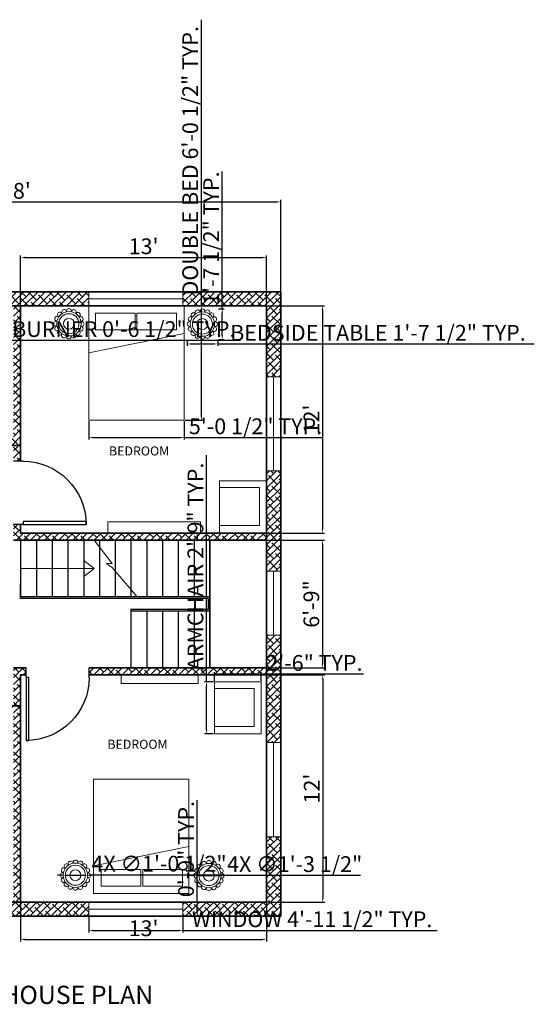
# Model space of a CAD drawing. Units: inches. Extents: x 1501 to 2163, y 1105 to 1729.
# Tile 2 of 2: x 1837 to 2163, y 1105 to 1729. Entities that reach past the tile are written whole.
import ezdxf

# ---------------------------------------------------------------- set-up
doc = ezdxf.new("R2010")
doc.units = ezdxf.units.IN
for name, color, linetype, lineweight in [('A-ANNO-DIMS', 2, 'Continuous', 18), ('A-ANNO-SYMB', 7, 'Continuous', 18), ('A-ANNO-TEXT', 7, 'Continuous', 18), ('A-AREA-IDEN', 7, 'Continuous', 18), ('A-DOOR', 3, 'Continuous', 25), ('A-FLOR-STRS', 7, 'Continuous', 25), ('A-GLAZ', 4, 'Continuous', 18), ('A-WALL', 7, 'Continuous', 35), ('A-WALL-PATT', 252, 'Continuous', 13), ('fur', 130, 'Continuous', 18)]:
    doc.layers.add(name, color=color, linetype=linetype, lineweight=lineweight)
doc.styles.get("Standard").update_dxf_attribs({"font": 'arial.ttf'})
doc.dimstyles.new('ISO-25', dxfattribs={"dimtxt": 10, "dimasz": 2.5, "dimexe": 1.25, "dimexo": 0.625, "dimtad": 1, "dimdec": 0, "dimlunit": 4, "dimtxsty": 'Standard', "dimcen": 2.5, "dimadec": 0, "dimazin": 0, "dimtfac": 1, "dimtdec": 0, "dimtmove": 0, "dimatfit": 3, "dimfxl": 1, "dimarcsym": 0})

# ---------------------------------------------------------------- blocks, each defined once
blk = doc.blocks.new('*U2')
for p, q in [((0, 0), (0, -6)), ((40, 0), (40, -6))]:
    blk.add_line(p, q)
blk.add_lwpolyline([(0, 0), (0, 40), (1.75, 40), (1.75, 0)], close=True)
blk.add_arc((0, 0), 40, 0, 90)
blk = doc.blocks.new('*D12')
at = {"layer": 'A-ANNO-DIMS', "color": 0, "lineweight": -2, "transparency": 16777216}
for p, q in [((1666.55, 1557.41), (1666.55, 1614.95)), ((1669.05, 1613.7), (2000.05, 1613.7)), ((2002.55, 1557.41), (2002.55, 1614.95))]:
    blk.add_line(p, q, dxfattribs=at)
at = {"layer": 'A-ANNO-DIMS', "color": 0, "lineweight": 100, "transparency": 16777216}
for points in [[(1669.05, 1614.12), (1669.05, 1613.29), (1666.55, 1613.7)], [(2000.05, 1614.12), (2000.05, 1613.29), (2002.55, 1613.7)]]:
    blk.add_solid(points, dxfattribs=at)
at = {"layer": 'Defpoints', "color": 0, "lineweight": 100, "transparency": 16777216}
for p in [(2002.55, 1613.7), (1666.55, 1556.78), (2002.55, 1556.78)]:
    blk.add_point(p, dxfattribs=at)
at = {"layer": 'A-ANNO-DIMS', "color": 0, "transparency": 16777216, "insert": (1834.55, 1619.44), "char_height": 10, "attachment_point": 5}
blk.add_mtext("28'", dxfattribs=at)
blk = doc.blocks.new('*D15')
at = {"layer": 'A-ANNO-DIMS', "color": 0, "lineweight": -2, "transparency": 16777216}
for p, q in [((1837.55, 1548.41), (1837.55, 1579.79)), ((1993.55, 1548.41), (1993.55, 1579.79)), ((1840.05, 1578.54), (1991.05, 1578.54))]:
    blk.add_line(p, q, dxfattribs=at)
at = {"layer": 'A-ANNO-DIMS', "color": 0, "lineweight": 100, "transparency": 16777216}
for points in [[(1840.05, 1578.95), (1840.05, 1578.12), (1837.55, 1578.54)], [(1991.05, 1578.95), (1991.05, 1578.12), (1993.55, 1578.54)]]:
    blk.add_solid(points, dxfattribs=at)
at = {"layer": 'Defpoints', "color": 0, "lineweight": 100, "transparency": 16777216}
for p in [(1993.55, 1578.54), (1837.55, 1547.78), (1993.55, 1547.78)]:
    blk.add_point(p, dxfattribs=at)
at = {"layer": 'A-ANNO-DIMS', "color": 0, "transparency": 16777216, "insert": (1915.55, 1584.27), "char_height": 10, "attachment_point": 5}
blk.add_mtext("13'", dxfattribs=at)
blk = doc.blocks.new('*D16')
at = {"layer": 'A-ANNO-DIMS', "color": 0, "lineweight": -2, "transparency": 16777216}
for p, q in [((1994.18, 1547.78), (2030.26, 1547.78)), ((2029.01, 1545.28), (2029.01, 1406.28)), ((1994.18, 1403.78), (2030.26, 1403.78))]:
    blk.add_line(p, q, dxfattribs=at)
at = {"layer": 'A-ANNO-DIMS', "color": 0, "lineweight": 100, "transparency": 16777216}
for points in [[(2028.6, 1545.28), (2029.43, 1545.28), (2029.01, 1547.78)], [(2028.6, 1406.28), (2029.43, 1406.28), (2029.01, 1403.78)]]:
    blk.add_solid(points, dxfattribs=at)
at = {"layer": 'Defpoints', "color": 0, "lineweight": 100, "transparency": 16777216}
for p in [(1993.55, 1547.78), (1993.55, 1403.78), (2029.01, 1403.78)]:
    blk.add_point(p, dxfattribs=at)
at = {"layer": 'A-ANNO-DIMS', "color": 0, "transparency": 16777216, "insert": (2023.37, 1475.78), "char_height": 10, "attachment_point": 5, "rotation": 90}
blk.add_mtext("12'", dxfattribs=at)
blk = doc.blocks.new('*D17')
at = {"layer": 'A-ANNO-DIMS', "color": 0, "lineweight": -2, "transparency": 16777216}
for p, q in [((1994.18, 1399.28), (2030.26, 1399.28)), ((2029.01, 1396.78), (2029.01, 1320.78)), ((1994.18, 1318.28), (2030.26, 1318.28))]:
    blk.add_line(p, q, dxfattribs=at)
at = {"layer": 'A-ANNO-DIMS', "color": 0, "lineweight": 100, "transparency": 16777216}
for points in [[(2028.59, 1396.78), (2029.43, 1396.78), (2029.01, 1399.28)], [(2028.59, 1320.78), (2029.43, 1320.78), (2029.01, 1318.28)]]:
    blk.add_solid(points, dxfattribs=at)
at = {"layer": 'Defpoints', "color": 0, "lineweight": 100, "transparency": 16777216}
for p in [(1993.55, 1399.28), (1993.55, 1318.28), (2029.01, 1318.28)]:
    blk.add_point(p, dxfattribs=at)
at = {"layer": 'A-ANNO-DIMS', "color": 0, "transparency": 16777216, "insert": (2023.28, 1358.78), "char_height": 10, "attachment_point": 5, "rotation": 90}
blk.add_mtext('6\'-9"', dxfattribs=at)
blk = doc.blocks.new('*D18')
at = {"layer": 'A-ANNO-DIMS', "color": 0, "lineweight": -2, "transparency": 16777216}
for p, q in [((1994.18, 1313.78), (2030.47, 1313.78)), ((2029.22, 1311.28), (2029.22, 1172.28)), ((1994.18, 1169.78), (2030.47, 1169.78))]:
    blk.add_line(p, q, dxfattribs=at)
at = {"layer": 'A-ANNO-DIMS', "color": 0, "lineweight": 100, "transparency": 16777216}
for points in [[(2028.8, 1311.28), (2029.64, 1311.28), (2029.22, 1313.78)], [(2028.8, 1172.28), (2029.64, 1172.28), (2029.22, 1169.78)]]:
    blk.add_solid(points, dxfattribs=at)
at = {"layer": 'Defpoints', "color": 0, "lineweight": 100, "transparency": 16777216}
for p in [(1993.55, 1313.78), (1993.55, 1169.78), (2029.22, 1169.78)]:
    blk.add_point(p, dxfattribs=at)
at = {"layer": 'A-ANNO-DIMS', "color": 0, "transparency": 16777216, "insert": (2023.57, 1241.78), "char_height": 10, "attachment_point": 5, "rotation": 90}
blk.add_mtext("12'", dxfattribs=at)
blk = doc.blocks.new('*D19')
at = {"layer": 'A-ANNO-DIMS', "color": 0, "lineweight": -2, "transparency": 16777216}
for p, q in [((1837.55, 1169.16), (1837.55, 1144.9)), ((1993.55, 1169.16), (1993.55, 1144.9)), ((1840.05, 1146.15), (1991.05, 1146.15))]:
    blk.add_line(p, q, dxfattribs=at)
at = {"layer": 'A-ANNO-DIMS', "color": 0, "lineweight": 100, "transparency": 16777216}
for points in [[(1840.05, 1146.57), (1840.05, 1145.74), (1837.55, 1146.15)], [(1991.05, 1146.57), (1991.05, 1145.74), (1993.55, 1146.15)]]:
    blk.add_solid(points, dxfattribs=at)
at = {"layer": 'Defpoints', "color": 0, "lineweight": 100, "transparency": 16777216}
for p in [(1837.55, 1169.78), (1993.55, 1169.78), (1993.55, 1146.15)]:
    blk.add_point(p, dxfattribs=at)
at = {"layer": 'A-ANNO-DIMS', "color": 0, "transparency": 16777216, "insert": (1915.55, 1151.89), "char_height": 10, "attachment_point": 5}
blk.add_mtext("13'", dxfattribs=at)
blk = doc.blocks.new('WIN-60IN')
blk.add_line((0, 4.5), (59.67, 4.5))
blk.add_lwpolyline([(0, 9), (59.67, 9), (59.67, 0), (0, 0)], close=True)
blk = doc.blocks.new('WIN-41IN')
blk.add_line((4.5, 0), (4.5, 40.59))
blk.add_lwpolyline([(0, 0), (9, 0), (9, 40.59), (0, 40.59)], close=True)
blk = doc.blocks.new('BED-DOUBLE')
blk.add_line((60.45, 55.13), (0, 42.75))
for points in [[(0, 72.55), (60.45, 72.55), (60.45, 0), (0, 0)], [(4.14, 68.02), (29.3, 68.02), (29.3, 57.38), (4.14, 57.38)], [(30.41, 68.02), (55.57, 68.02), (55.57, 57.38), (30.41, 57.38)]]:
    blk.add_lwpolyline(points, close=True)
blk = doc.blocks.new('CHAIR-ARM')
for p, q in [((0, 28.77), (25.27, 28.77)), ((25.27, 28.77), (25.27, 4.77)), ((25.27, 4.77), (0, 4.77))]:
    blk.add_line(p, q)
blk.add_lwpolyline([(29.77, 0), (0, 0), (0, 33.02), (29.77, 33.02)], close=True)
blk = doc.blocks.new('*U4')
at = {"layer": 'fur'}
blk.add_arc((0, -0.52), 1.52, 341.57303, 197.79701, dxfattribs=at)
blk = doc.blocks.new('*U5')
at = {"layer": 'fur', "transparency": 16777216}
for p, rotation in [((1949.32, 1541.68), 45), ((1952.12, 1543.53), 22.49999999999997), ((1958.69, 1543.49), 337.5), ((1961.46, 1541.62), 315), ((1946.77, 1535.62), 90), ((1947.44, 1538.9), 67.49999999999997), ((1963.31, 1538.82), 292.5), ((1963.95, 1535.53), 269.9999999999999), ((1947.41, 1532.33), 112.5), ((1949.26, 1529.53), 134.9999999999999), ((1961.4, 1529.47), 225), ((1963.28, 1532.25), 247.5), ((1952.03, 1527.66), 157.5), ((1955.32, 1526.99), 180), ((1958.61, 1527.62), 202.4999999999999)]:
    blk.add_blockref('*U4', p, dxfattribs=dict(at, rotation=rotation))
blk.add_blockref('*U4', (1955.41, 1544.16), dxfattribs=at)
blk = doc.blocks.new('BEDSIDE-ROUND')
for radius in [7.73, 7.73, 7.73, 6.37, 3.47]:
    blk.add_circle((9.59, 9.59), radius)
blk.add_blockref('*U5', (-1945.77, -1525.99))
blk = doc.blocks.new('*D32')
at = {"layer": 'A-ANNO-DIMS', "color": 0, "lineweight": -2, "transparency": 16777216}
for p, q in [((1880.88, 1160.16), (1880.88, 1150.58)), ((1940.55, 1160.16), (1940.55, 1150.58)), ((1883.38, 1151.83), (1938.05, 1151.83)), ((1940.55, 1151.83), (2101.92, 1151.83))]:
    blk.add_line(p, q, dxfattribs=at)
at = {"layer": 'A-ANNO-DIMS', "color": 0, "lineweight": 100, "transparency": 16777216}
for points in [[(1883.38, 1152.25), (1883.38, 1151.42), (1880.88, 1151.83)], [(1938.05, 1152.25), (1938.05, 1151.42), (1940.55, 1151.83)]]:
    blk.add_solid(points, dxfattribs=at)
at = {"layer": 'Defpoints', "color": 0, "lineweight": 100, "transparency": 16777216}
for p in [(1880.88, 1160.78), (1940.55, 1160.78), (1940.55, 1151.83)]:
    blk.add_point(p, dxfattribs=at)
at = {"layer": 'A-ANNO-DIMS', "color": 0, "transparency": 16777216, "insert": (2022.48, 1157.63), "char_height": 10, "attachment_point": 5}
blk.add_mtext('WINDOW 4\'-11 1/2" TYP.', dxfattribs=at)
blk = doc.blocks.new('*D33')
at = {"layer": 'A-ANNO-DIMS', "color": 0, "lineweight": -2, "transparency": 16777216}
for p, q in [((1949.5, 1169.78), (1949.5, 1234.49)), ((1941.18, 1169.78), (1950.75, 1169.78)), ((1949.5, 1163.28), (1949.5, 1167.28)), ((1941.18, 1160.78), (1950.75, 1160.78))]:
    blk.add_line(p, q, dxfattribs=at)
at = {"layer": 'A-ANNO-DIMS', "color": 0, "lineweight": 100, "transparency": 16777216}
for points in [[(1949.09, 1167.28), (1949.92, 1167.28), (1949.5, 1169.78)], [(1949.09, 1163.28), (1949.92, 1163.28), (1949.5, 1160.78)]]:
    blk.add_solid(points, dxfattribs=at)
at = {"layer": 'Defpoints', "color": 0, "lineweight": 100, "transparency": 16777216}
for p in [(1940.55, 1169.78), (1949.5, 1169.78), (1940.55, 1160.78)]:
    blk.add_point(p, dxfattribs=at)
at = {"layer": 'A-ANNO-DIMS', "color": 0, "transparency": 16777216, "insert": (1943.77, 1203.39), "char_height": 10, "attachment_point": 5, "rotation": 90}
blk.add_mtext('0\'-9" TYP.', dxfattribs=at)
blk = doc.blocks.new('*D38')
at = {"layer": 'A-ANNO-DIMS', "color": 0, "lineweight": -2, "transparency": 16777216}
for p, q in [((1955.54, 1309.46), (1955.54, 1453.14)), ((1959.87, 1309.46), (1954.29, 1309.46)), ((1955.54, 1278.94), (1955.54, 1306.96)), ((1959.87, 1276.44), (1954.29, 1276.44))]:
    blk.add_line(p, q, dxfattribs=at)
at = {"layer": 'A-ANNO-DIMS', "color": 0, "lineweight": 100, "transparency": 16777216}
for points in [[(1955.12, 1306.96), (1955.96, 1306.96), (1955.54, 1309.46)], [(1955.12, 1278.94), (1955.96, 1278.94), (1955.54, 1276.44)]]:
    blk.add_solid(points, dxfattribs=at)
at = {"layer": 'Defpoints', "color": 0, "lineweight": 100, "transparency": 16777216}
for p in [(1955.54, 1309.46), (1960.49, 1309.46), (1960.49, 1276.44)]:
    blk.add_point(p, dxfattribs=at)
at = {"layer": 'A-ANNO-DIMS', "color": 0, "transparency": 16777216, "insert": (1949.74, 1382.55), "char_height": 10, "attachment_point": 5, "rotation": 90}
blk.add_mtext('ARMCHAIR 2\'-9" TYP.', dxfattribs=at)
blk = doc.blocks.new('*D39')
at = {"layer": 'A-ANNO-DIMS', "color": 0, "lineweight": -2, "transparency": 16777216}
for p, q in [((1960.49, 1310.09), (1960.49, 1315.66)), ((1962.99, 1314.41), (1987.76, 1314.41)), ((1990.26, 1310.09), (1990.26, 1315.66)), ((1990.26, 1314.41), (2055.14, 1314.41))]:
    blk.add_line(p, q, dxfattribs=at)
at = {"layer": 'A-ANNO-DIMS', "color": 0, "lineweight": 100, "transparency": 16777216}
for points in [[(1962.99, 1314.83), (1962.99, 1314), (1960.49, 1314.41)], [(1987.76, 1314.83), (1987.76, 1314), (1990.26, 1314.41)]]:
    blk.add_solid(points, dxfattribs=at)
at = {"layer": 'Defpoints', "color": 0, "lineweight": 100, "transparency": 16777216}
for p in [(1990.26, 1314.41), (1960.49, 1309.46), (1990.26, 1309.46)]:
    blk.add_point(p, dxfattribs=at)
at = {"layer": 'A-ANNO-DIMS', "color": 0, "transparency": 16777216, "insert": (2023.95, 1320.14), "char_height": 10, "attachment_point": 5}
blk.add_mtext('2\'-6" TYP.', dxfattribs=at)
blk = doc.blocks.new('*D40')
at = {"layer": 'A-ANNO-DIMS', "color": 0, "lineweight": -2, "transparency": 16777216}
for p, q in [((1943.18, 1525.92), (1943.18, 1522.39)), ((1945.68, 1523.64), (1960.06, 1523.64)), ((1962.56, 1525.92), (1962.56, 1522.39)), ((1962.56, 1523.64), (2163.47, 1523.64))]:
    blk.add_line(p, q, dxfattribs=at)
at = {"layer": 'A-ANNO-DIMS', "color": 0, "lineweight": 100, "transparency": 16777216}
for points in [[(1945.68, 1524.05), (1945.68, 1523.22), (1943.18, 1523.64)], [(1960.06, 1524.05), (1960.06, 1523.22), (1962.56, 1523.64)]]:
    blk.add_solid(points, dxfattribs=at)
at = {"layer": 'Defpoints', "color": 0, "lineweight": 100, "transparency": 16777216}
for p in [(1943.18, 1526.54), (1962.56, 1526.54), (1962.56, 1523.64)]:
    blk.add_point(p, dxfattribs=at)
at = {"layer": 'A-ANNO-DIMS', "color": 0, "transparency": 16777216, "insert": (2064.26, 1529.43), "char_height": 10, "attachment_point": 5}
blk.add_mtext('BEDSIDE TABLE 1\'-7 1/2" TYP.', dxfattribs=at)
blk = doc.blocks.new('*D41')
at = {"layer": 'A-ANNO-DIMS', "color": 0, "lineweight": -2, "transparency": 16777216}
for p, q in [((1965.46, 1545.92), (1965.46, 1632.98)), ((1963.18, 1545.92), (1966.71, 1545.92)), ((1965.46, 1529.04), (1965.46, 1543.42)), ((1963.18, 1526.54), (1966.71, 1526.54))]:
    blk.add_line(p, q, dxfattribs=at)
at = {"layer": 'A-ANNO-DIMS', "color": 0, "lineweight": 100, "transparency": 16777216}
for points in [[(1965.04, 1543.42), (1965.88, 1543.42), (1965.46, 1545.92)], [(1965.04, 1529.04), (1965.88, 1529.04), (1965.46, 1526.54)]]:
    blk.add_solid(points, dxfattribs=at)
at = {"layer": 'Defpoints', "color": 0, "lineweight": 100, "transparency": 16777216}
for p in [(1962.56, 1545.92), (1965.46, 1545.92), (1962.56, 1526.54)]:
    blk.add_point(p, dxfattribs=at)
at = {"layer": 'A-ANNO-DIMS', "color": 0, "transparency": 16777216, "insert": (1959.67, 1590.7), "char_height": 10, "attachment_point": 5, "rotation": 90}
blk.add_mtext('1\'-7 1/2" TYP.', dxfattribs=at)
blk = doc.blocks.new('*D42')
at = {"layer": 'A-ANNO-DIMS', "color": 0, "lineweight": -2, "transparency": 16777216}
for p, q in [((1952.22, 1547.78), (1952.22, 1729.23)), ((1941.96, 1547.78), (1953.47, 1547.78)), ((1952.22, 1477.73), (1952.22, 1545.28)), ((1941.96, 1475.23), (1953.47, 1475.23))]:
    blk.add_line(p, q, dxfattribs=at)
at = {"layer": 'A-ANNO-DIMS', "color": 0, "lineweight": 100, "transparency": 16777216}
for points in [[(1951.8, 1545.28), (1952.63, 1545.28), (1952.22, 1547.78)], [(1951.8, 1477.73), (1952.63, 1477.73), (1952.22, 1475.23)]]:
    blk.add_solid(points, dxfattribs=at)
at = {"layer": 'Defpoints', "color": 0, "lineweight": 100, "transparency": 16777216}
for p in [(1941.33, 1547.78), (1952.22, 1547.78), (1941.33, 1475.23)]:
    blk.add_point(p, dxfattribs=at)
at = {"layer": 'A-ANNO-DIMS', "color": 0, "transparency": 16777216, "insert": (1946.42, 1639.76), "char_height": 10, "attachment_point": 5, "rotation": 90}
blk.add_mtext('DOUBLE BED 6\'-0 1/2" TYP.', dxfattribs=at)
blk = doc.blocks.new('*D43')
at = {"layer": 'A-ANNO-DIMS', "color": 0, "lineweight": -2, "transparency": 16777216}
for p, q in [((1880.88, 1474.61), (1880.88, 1463.1)), ((1941.33, 1474.61), (1941.33, 1463.1)), ((1883.38, 1464.35), (1938.83, 1464.35)), ((1941.33, 1464.35), (2029.34, 1464.35))]:
    blk.add_line(p, q, dxfattribs=at)
at = {"layer": 'A-ANNO-DIMS', "color": 0, "lineweight": 100, "transparency": 16777216}
for points in [[(1883.38, 1464.77), (1883.38, 1463.93), (1880.88, 1464.35)], [(1938.83, 1464.77), (1938.83, 1463.93), (1941.33, 1464.35)]]:
    blk.add_solid(points, dxfattribs=at)
at = {"layer": 'Defpoints', "color": 0, "lineweight": 100, "transparency": 16777216}
for p in [(1880.88, 1475.23), (1941.33, 1475.23), (1941.33, 1464.35)]:
    blk.add_point(p, dxfattribs=at)
at = {"layer": 'A-ANNO-DIMS', "color": 0, "transparency": 16777216, "insert": (1986.59, 1470.15), "char_height": 10, "attachment_point": 5}
blk.add_mtext('5\'-0 1/2" TYP.', dxfattribs=at)
blk = doc.blocks.new('*D44')
at = {"layer": 'A-ANNO-DIMS', "color": 0, "lineweight": -2, "transparency": 16777216}
for p, q in [((1820, 1526.33), (1820, 1524.73)), ((1822.5, 1525.98), (1824.03, 1525.98)), ((1826.53, 1526.33), (1826.53, 1524.73)), ((1826.53, 1525.98), (1976.97, 1525.98))]:
    blk.add_line(p, q, dxfattribs=at)
at = {"layer": 'A-ANNO-DIMS', "color": 0, "lineweight": 100, "transparency": 16777216}
for points in [[(1822.5, 1526.39), (1822.5, 1525.56), (1820, 1525.98)], [(1824.03, 1526.39), (1824.03, 1525.56), (1826.53, 1525.98)]]:
    blk.add_solid(points, dxfattribs=at)
at = {"layer": 'Defpoints', "color": 0, "lineweight": 100, "transparency": 16777216}
for p in [(1820, 1526.95), (1826.53, 1526.95), (1826.53, 1525.98)]:
    blk.add_point(p, dxfattribs=at)
at = {"layer": 'A-ANNO-DIMS', "color": 0, "transparency": 16777216, "insert": (1903, 1531.77), "char_height": 10, "attachment_point": 5}
blk.add_mtext('BURNER 0\'-6 1/2" TYP.', dxfattribs=at)
blk = doc.blocks.new('*D45')
at = {"layer": 'A-ANNO-DIMS', "color": 0, "lineweight": -2, "transparency": 16777216}
for p, q in [((1827.51, 1533.48), (1827.51, 1621.49)), ((1827.16, 1533.48), (1828.76, 1533.48)), ((1827.51, 1529.45), (1827.51, 1530.98)), ((1827.16, 1526.95), (1828.76, 1526.95))]:
    blk.add_line(p, q, dxfattribs=at)
at = {"layer": 'A-ANNO-DIMS', "color": 0, "lineweight": 100, "transparency": 16777216}
for points in [[(1827.1, 1530.98), (1827.93, 1530.98), (1827.51, 1533.48)], [(1827.1, 1529.45), (1827.93, 1529.45), (1827.51, 1526.95)]]:
    blk.add_solid(points, dxfattribs=at)
at = {"layer": 'Defpoints', "color": 0, "lineweight": 100, "transparency": 16777216}
for p in [(1826.53, 1533.48), (1827.51, 1533.48), (1826.53, 1526.95)]:
    blk.add_point(p, dxfattribs=at)
at = {"layer": 'A-ANNO-DIMS', "color": 0, "transparency": 16777216, "insert": (1821.72, 1578.74), "char_height": 10, "attachment_point": 5, "rotation": 90}
blk.add_mtext('0\'-6 1/2" TYP.', dxfattribs=at)
blk = doc.blocks.new('*D51')
at = {"layer": 'A-ANNO-DIMS', "color": 0, "lineweight": -2, "transparency": 16777216}
for p, q in [((1946.77, 1186.58), (1944.27, 1186.59)), ((1949.27, 1186.58), (1964.73, 1186.58)), ((2053.1, 1186.56), (1967.23, 1186.58))]:
    blk.add_line(p, q, dxfattribs=at)
at = {"layer": 'A-ANNO-DIMS', "color": 0, "lineweight": 100, "transparency": 16777216}
for points in [[(1946.77, 1187), (1946.77, 1186.17), (1949.27, 1186.58)], [(1967.23, 1187), (1967.23, 1186.16), (1964.73, 1186.58)]]:
    blk.add_solid(points, dxfattribs=at)
at = {"layer": 'Defpoints', "color": 0, "lineweight": 100, "transparency": 16777216}
for p in [(1949.27, 1186.58), (1964.73, 1186.58)]:
    blk.add_point(p, dxfattribs=at)
at = {"layer": 'A-ANNO-DIMS', "color": 0, "transparency": 16777216, "insert": (2011.42, 1192.58), "char_height": 10, "attachment_point": 5, "rotation": 359.98576}
blk.add_mtext('4X ∅1\'-3 1/2"', dxfattribs=at)
blk = doc.blocks.new('*D52')
at = {"layer": 'A-ANNO-DIMS', "color": 0, "lineweight": -2, "transparency": 16777216}
for p, q in [((1863.44, 1186.82), (1860.94, 1186.82)), ((1865.94, 1186.82), (1878.67, 1186.82)), ((1967.04, 1186.82), (1881.17, 1186.82))]:
    blk.add_line(p, q, dxfattribs=at)
at = {"layer": 'A-ANNO-DIMS', "color": 0, "lineweight": 100, "transparency": 16777216}
for points in [[(1863.44, 1187.23), (1863.44, 1186.4), (1865.94, 1186.82)], [(1881.17, 1187.23), (1881.17, 1186.4), (1878.67, 1186.82)]]:
    blk.add_solid(points, dxfattribs=at)
at = {"layer": 'Defpoints', "color": 0, "lineweight": 100, "transparency": 16777216}
for p in [(1865.94, 1186.82), (1878.67, 1186.82)]:
    blk.add_point(p, dxfattribs=at)
at = {"layer": 'A-ANNO-DIMS', "color": 0, "transparency": 16777216, "insert": (1925.36, 1192.83), "char_height": 10, "attachment_point": 5, "rotation": 359.99936}
blk.add_mtext('4X ∅1\'-0 1/2"', dxfattribs=at)

msp = doc.modelspace()

# ---------------------------------------------------------------- hatches: boundary and pattern name
at = {"layer": 'A-WALL-PATT'}
h = msp.add_hatch(dxfattribs=at)
h.set_pattern_fill('ANSI38', color=256)
h.paths.add_polyline_path([(1748.43, 1556.78), (1666.55, 1556.78), (1666.55, 1522.79), (1675.55, 1522.79), (1675.55, 1547.78), (1748.43, 1547.78)])
h.paths.add_polyline_path([(1880.88, 1556.78), (1808.1, 1556.78), (1808.1, 1547.78), (1880.88, 1547.78)])
h.paths.add_polyline_path([(2002.55, 1556.78), (1940.55, 1556.78), (1940.55, 1547.78), (1993.55, 1547.78), (1993.55, 1502.88), (2002.55, 1502.88)])
h.paths.add_polyline_path([(1675.55, 1482.19), (1666.55, 1482.19), (1666.55, 1456.67), (1675.55, 1456.67)])
h.paths.add_polyline_path([(1675.55, 1321.98), (1666.55, 1321.98), (1666.55, 1160.78), (1675.55, 1160.78), (1675.55, 1169.78)])
h.paths.add_polyline_path([(1778.68, 1293.45), (1778.68, 1294.28), (1675.55, 1294.28), (1675.55, 1289.78), (1778.68, 1289.78)])
h.paths.add_polyline_path([(1675.55, 1406.78), (1675.55, 1416.08), (1666.55, 1416.08), (1666.55, 1381.65), (1675.55, 1381.65)])
h = msp.add_hatch(dxfattribs=at)
h.set_pattern_fill('ANSI38', color=256)
h.paths.add_polyline_path([(1728.05, 1510.56), (1723.55, 1510.56), (1723.55, 1463.78), (1728.05, 1463.78)])
h.paths.add_polyline_path([(1728.05, 1463.28), (1728.05, 1463.78), (1723.55, 1463.78), (1675.55, 1463.78), (1675.55, 1459.28), (1728.05, 1459.28)])
h.paths.add_polyline_path([(1728.05, 1459.28), (1723.55, 1459.28), (1723.55, 1415.28), (1723.55, 1411.28), (1720.31, 1411.28), (1720.31, 1406.78), (1728.05, 1406.78)])
h.paths.add_polyline_path([(1789.9, 1463.78), (1728.05, 1463.78), (1728.05, 1463.28), (1728.05, 1459.28), (1789.9, 1459.28)])
h.paths.add_polyline_path([(1837.55, 1547.78), (1833.05, 1547.78), (1833.05, 1523.78), (1833.05, 1459.28), (1837.55, 1459.28)])
h.paths.add_polyline_path([(1833.05, 1463.78), (1829.9, 1463.78), (1829.9, 1459.28), (1833.05, 1459.28)])
h.paths.add_polyline_path([(1837.55, 1459.28), (1833.05, 1459.28), (1833.05, 1449.28), (1837.55, 1449.28)])
h.paths.add_polyline_path([(2002.55, 1443.21), (1993.55, 1443.21), (1993.55, 1379.58), (2002.55, 1379.58)])
h.paths.add_polyline_path([(2002.55, 1338.99), (1993.55, 1338.99), (1993.55, 1270.9), (2002.55, 1270.9)])
h.paths.add_polyline_path([(1993.55, 1318.28), (1957.55, 1318.28), (1881.07, 1318.28), (1881.07, 1313.78), (1993.55, 1313.78)])
h.paths.add_polyline_path([(2002.55, 1211.23), (1993.55, 1211.23), (1993.55, 1169.78), (1940.55, 1169.78), (1940.55, 1160.78), (2002.55, 1160.78)])
h.paths.add_polyline_path([(1880.88, 1169.78), (1817.84, 1169.78), (1817.84, 1160.78), (1880.88, 1160.78)])
h = msp.add_hatch(dxfattribs=at)
h.set_pattern_fill('ANSI38', color=256)
h.paths.add_polyline_path([(1993.55, 1403.78), (1870.74, 1403.78), (1837.55, 1403.78), (1837.55, 1409.28), (1833.05, 1409.28), (1833.05, 1399.28), (1993.55, 1399.28)])
h.paths.add_polyline_path([(1837.55, 1294.28), (1827.53, 1294.28), (1827.53, 1293.45), (1827.53, 1289.78), (1833.05, 1289.78), (1833.05, 1169.78), (1837.55, 1169.78)])
h.paths.add_polyline_path([(1837.55, 1313.78), (1841.07, 1313.78), (1841.07, 1318.28), (1833.05, 1318.28), (1833.05, 1294.28), (1837.55, 1294.28)])

# ---------------------------------------------------------------- linework, layer by layer
at = {"layer": 'A-ANNO-SYMB'}
for p, q in [((1884.24, 1399.28), (1895.54, 1384.52)), ((1884.27, 1381.28), (1877.55, 1386.32)), ((1837.55, 1381.28), (1884.27, 1381.28)), ((1884.27, 1381.28), (1877.55, 1376.24)), ((1895.54, 1384.52), (1891.77, 1384.52)), ((1891.77, 1384.52), (1895.41, 1382.05)), ((1895.41, 1382.05), (1911.38, 1363.28))]:
    msp.add_line(p, q, dxfattribs=at)
at = {"layer": 'A-FLOR-STRS'}
for p, q in [((1837.55, 1399.28), (1837.55, 1363.28)), ((1847.55, 1399.28), (1847.55, 1363.28)), ((1857.55, 1399.28), (1857.55, 1363.28)), ((1867.55, 1399.28), (1867.55, 1363.28)), ((1877.55, 1399.28), (1877.55, 1363.28)), ((1887.55, 1399.28), (1887.55, 1363.28)), ((1897.55, 1399.28), (1897.55, 1363.28)), ((1907.55, 1399.28), (1907.55, 1363.28)), ((1917.55, 1399.28), (1917.55, 1363.28)), ((1927.55, 1399.28), (1927.55, 1363.28)), ((1937.55, 1399.28), (1937.55, 1363.28)), ((1947.55, 1399.28), (1947.55, 1363.28)), ((1957.55, 1318.28), (1957.55, 1399.28)), ((1957.55, 1399.28), (1957.55, 1318.28)), ((1837.55, 1362.28), (1837.55, 1371.74)), ((1957.55, 1363.28), (1837.55, 1363.28)), ((1956.55, 1362.28), (1837.55, 1362.28)), ((1957.55, 1363.28), (1876.49, 1363.28)), ((1956.55, 1362.28), (1956.55, 1355.28)), ((1957.55, 1363.28), (1957.55, 1354.28)), ((1956.55, 1355.28), (1907.55, 1355.28)), ((1907.55, 1355.28), (1907.55, 1348.77)), ((1957.55, 1354.28), (1907.55, 1354.28)), ((1907.55, 1354.28), (1907.55, 1318.28)), ((1917.55, 1354.28), (1917.55, 1318.28)), ((1927.55, 1354.28), (1927.55, 1318.28)), ((1937.55, 1354.28), (1937.55, 1318.28)), ((1947.55, 1354.28), (1947.55, 1318.28)), ((1957.55, 1318.28), (1957.55, 1354.28)), ((1993.55, 1318.28), (1957.55, 1318.28))]:
    msp.add_line(p, q, dxfattribs=at)
at = {"layer": 'A-WALL'}
for p, q in [((1666.55, 1556.78), (2002.55, 1556.78)), ((2002.55, 1556.78), (2002.55, 1160.78)), ((1837.55, 1547.78), (1837.55, 1459.28)), ((1837.55, 1547.78), (1837.55, 1449.28)), ((1837.55, 1459.28), (1829.9, 1459.28)), ((1837.55, 1409.28), (1837.55, 1403.78)), ((1833.05, 1399.28), (1993.55, 1399.28)), ((1837.55, 1403.78), (1993.55, 1403.78)), ((1870.74, 1403.78), (1993.55, 1403.78)), ((1841.07, 1318.28), (1833.05, 1318.28)), ((1993.55, 1318.28), (1881.07, 1318.28)), ((1837.55, 1294.28), (1837.55, 1313.78)), ((1841.07, 1313.78), (1837.55, 1313.78)), ((1993.55, 1313.78), (1881.07, 1313.78)), ((1993.55, 1169.78), (1993.55, 1313.78)), ((1826.46, 1294.28), (1837.55, 1294.28)), ((1837.55, 1169.78), (1837.55, 1294.28)), ((2002.55, 1160.78), (1817.84, 1160.78))]:
    msp.add_line(p, q, dxfattribs=at)
for points in [[(1675.55, 1160.78), (1666.55, 1160.78), (1666.55, 1556.78), (2002.55, 1556.78), (2002.55, 1160.78), (1817.84, 1160.78)], [(1675.55, 1169.78), (1675.55, 1547.78), (1993.55, 1547.78), (1993.55, 1169.78), (1817.84, 1169.78)]]:
    msp.add_lwpolyline(points, dxfattribs=at)
at = {"layer": 'fur'}
msp.add_line((1963.78, 1432.55), (1963.78, 1432.55), dxfattribs=at)
for points in [[(1892.95, 1403.78), (1951.72, 1403.78), (1951.72, 1410.8), (1892.95, 1410.8)], [(1901.29, 1313.78), (1950.21, 1313.78), (1950.21, 1308.29), (1901.29, 1308.29)]]:
    msp.add_lwpolyline(points, close=True, dxfattribs=at)

# ---------------------------------------------------------------- block references
at = {"layer": 'A-DOOR', "xscale": -1}
for p, rotation in [((1839.05, 1409.28), 270), ((1841.07, 1312.28), 180)]:
    msp.add_blockref('*U2', p, dxfattribs=dict(at, rotation=rotation))
at = {"layer": 'A-GLAZ'}
for name, p in [('WIN-60IN', (1880.88, 1547.79)), ('WIN-41IN', (1993.55, 1338.99)), ('WIN-60IN', (1880.88, 1160.79))]:
    msp.add_blockref(name, p, dxfattribs=at)
for p, rotation in [((1993.55, 1502.88), 269.9999999999991), ((1993.55, 1270.9), 269.9999999999989)]:
    msp.add_blockref('WIN-60IN', p, dxfattribs=dict(at, rotation=rotation))
at = {"layer": 'fur'}
for name, p in [('BEDSIDE-ROUND', (1858.58, 1526.88)), ('BED-DOUBLE', (1880.88, 1475.23)), ('BEDSIDE-ROUND', (1943.28, 1526.64)), ('CHAIR-ARM', (1963.78, 1403.79)), ('CHAIR-ARM', (1960.49, 1276.44))]:
    msp.add_blockref(name, p, dxfattribs=at)
at = {"layer": 'fur', "rotation": 180}
for name, p in [('BED-DOUBLE', (1944.29, 1247.81)), ('BEDSIDE-ROUND', (1881.89, 1196.41)), ('BEDSIDE-ROUND', (1966.59, 1196.17))]:
    msp.add_blockref(name, p, dxfattribs=at)

# ---------------------------------------------------------------- texts
at = {"layer": 'A-ANNO-TEXT', "insert": (1780.96, 1116.75), "char_height": 11.5661, "attachment_point": 1}
msp.add_mtext_dynamic_manual_height_columns('2BHK HOUSE PLAN', width=1377.2449, gutter_width=57.83, heights=[0], dxfattribs=at)
at = {"layer": 'A-AREA-IDEN', "char_height": 5.753, "attachment_point": 1}
for insert in [(1893.65, 1458.69), (1892.6, 1272.71)]:
    msp.add_mtext_dynamic_manual_height_columns('BEDROOM', width=61.1637, gutter_width=28.76, heights=[0], dxfattribs=dict(at, insert=insert))

# ---------------------------------------------------------------- dimensions: what is measured, and where the dimension line sits
at = {"layer": 'A-ANNO-DIMS'}
for base, p1, p2, text, picture, middle in [((1952.2155, 1547.7848), (1941.3327, 1475.2326), (1941.3327, 1547.7848), 'DOUBLE BED <> TYP.', '*D42', (1946.4166, 1639.757)), ((1965.46, 1545.92), (1962.56, 1526.54), (1962.56, 1545.92), '<> TYP.', '*D41', (1959.67, 1590.7)), ((1827.51, 1533.48), (1826.53, 1526.95), (1826.53, 1533.48), '<> TYP.', '*D45', (1821.72, 1578.74)), ((1955.54, 1309.46), (1960.49, 1276.44), (1960.49, 1309.46), 'ARMCHAIR <> TYP.', '*D38', (1949.74, 1382.55)), ((1949.5, 1169.78), (1940.55, 1160.78), (1940.55, 1169.78), '<> TYP.', '*D33', (1943.77, 1203.39))]:
    dim = msp.add_linear_dim(base=base, p1=p1, p2=p2, angle=90, text=text, dimstyle='ISO-25', override={"dimdec": 1, "dimlfac": 1, "dimrnd": 0, "dimzin": 1, "dimdsep": 46, "dimlunit": 4, "dimfrac": 2}, dxfattribs=at)
    dim.commit()
    dim.dimension.update_dxf_attribs({"geometry": picture, "text_midpoint": middle})
for base, p1, p2, picture, middle in [((2002.55, 1613.7), (1666.55, 1556.78), (2002.55, 1556.78), '*D12', (1834.55, 1619.44)), ((1993.55, 1578.54), (1837.55, 1547.78), (1993.55, 1547.78), '*D15', (1915.55, 1584.27)), ((1993.55, 1146.15), (1837.55, 1169.78), (1993.55, 1169.78), '*D19', (1915.55, 1151.89))]:
    dim = msp.add_linear_dim(base=base, p1=p1, p2=p2, dimstyle='ISO-25', override={"dimclrd": 0, "dimclre": 0, "dimclrt": 0}, dxfattribs=at)
    dim.commit()
    dim.dimension.update_dxf_attribs({"geometry": picture, "text_midpoint": middle})
for base, p1, p2, text, picture, middle in [((1962.56, 1523.64), (1943.18, 1526.54), (1962.56, 1526.54), 'BEDSIDE TABLE <> TYP.', '*D40', (2064.26, 1529.43)), ((1826.53, 1525.98), (1820, 1526.95), (1826.53, 1526.95), 'BURNER <> TYP.', '*D44', (1903, 1531.77)), ((1941.3327, 1464.3498), (1880.8843, 1475.2326), (1941.3327, 1475.2326), '<> TYP.', '*D43', (1986.5859, 1470.1453)), ((1990.26, 1314.41), (1960.49, 1309.46), (1990.26, 1309.46), '<> TYP.', '*D39', (2023.95, 1320.14)), ((1940.55, 1151.83), (1880.88, 1160.78), (1940.55, 1160.78), 'WINDOW <> TYP.', '*D32', (2022.48, 1157.63))]:
    dim = msp.add_linear_dim(base=base, p1=p1, p2=p2, text=text, dimstyle='ISO-25', override={"dimdec": 1, "dimlfac": 1, "dimrnd": 0, "dimzin": 1, "dimdsep": 46, "dimlunit": 4, "dimfrac": 2}, dxfattribs=at)
    dim.commit()
    dim.dimension.update_dxf_attribs({"geometry": picture, "text_midpoint": middle})
for base, p1, p2, picture, middle in [((2029.01, 1403.78), (1993.55, 1547.78), (1993.55, 1403.78), '*D16', (2023.37, 1475.78)), ((2029.01, 1318.28), (1993.55, 1399.28), (1993.55, 1318.28), '*D17', (2023.28, 1358.78)), ((2029.22, 1169.78), (1993.55, 1313.78), (1993.55, 1169.78), '*D18', (2023.57, 1241.78))]:
    dim = msp.add_linear_dim(base=base, p1=p1, p2=p2, angle=90, dimstyle='ISO-25', override={"dimclrd": 0, "dimclre": 0, "dimclrt": 0}, dxfattribs=at)
    dim.commit()
    dim.dimension.update_dxf_attribs({"geometry": picture, "text_midpoint": middle})
for p1, p2, picture, middle in [((1865.94, 1186.82), (1878.67, 1186.82), '*D52', (1925.36, 1186.82)), ((1949.27, 1186.58), (1964.73, 1186.58), '*D51', (2011.42, 1186.57))]:
    dim = msp.add_diameter_dim_2p(p1=p1, p2=p2, text='4X <>', dimstyle='ISO-25', override={"dimdec": 1, "dimlfac": 1, "dimrnd": 0, "dimzin": 1, "dimdsep": 46, "dimlunit": 4, "dimfrac": 2}, dxfattribs=at)
    dim.commit()
    dim.dimension.update_dxf_attribs({"geometry": picture, "text_midpoint": middle, "dimtype": 163})

doc.saveas('drawing.dxf')
